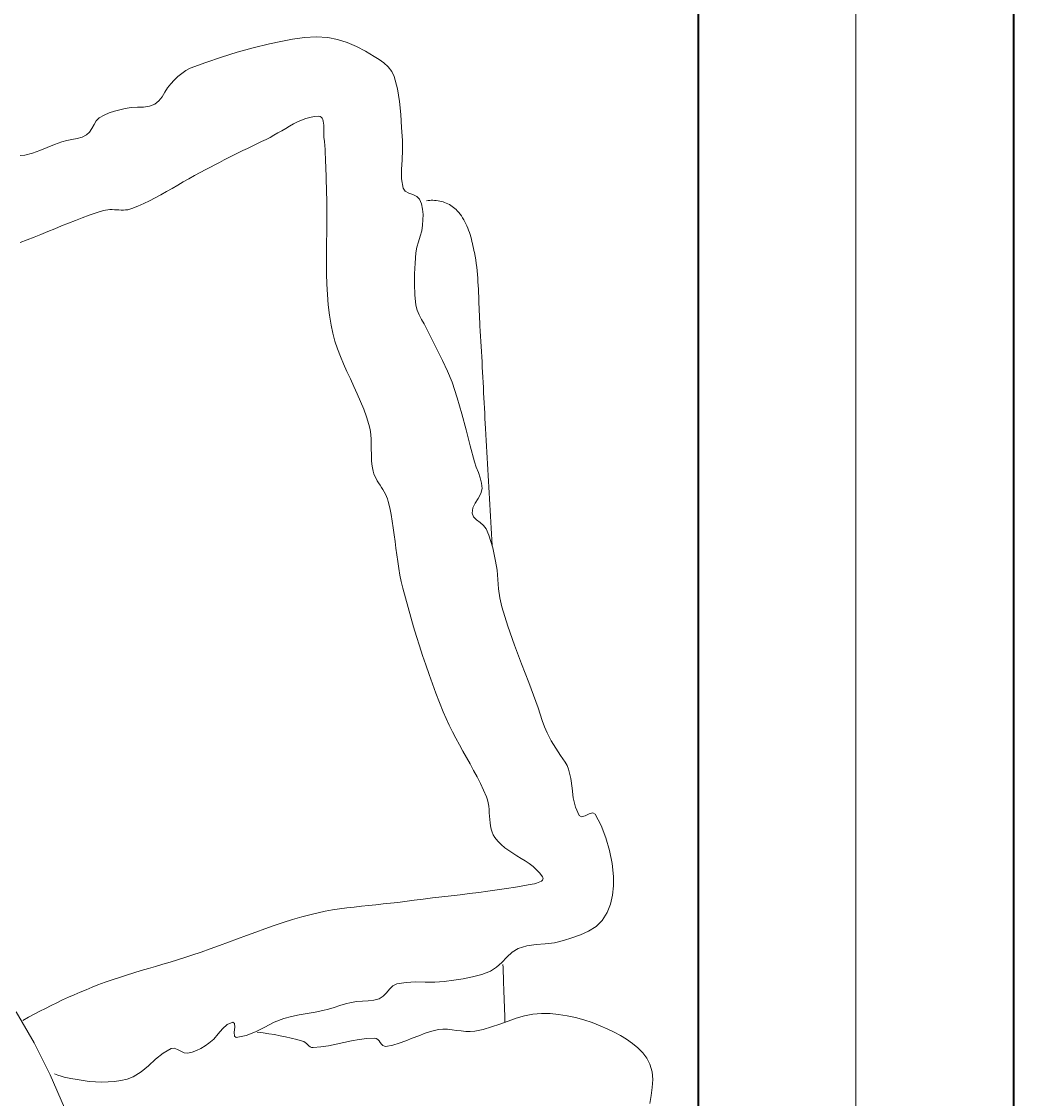
# Model space of a CAD drawing. Units: inches. Extents: x 1441 to 2460, y 1648 to 2683.
# Tile 18 of 35: x 1861 to 1890, y 2091 to 2122. Entities that reach past the tile are written whole.
import ezdxf

# ---------------------------------------------------------------- set-up
doc = ezdxf.new("R2010")
doc.units = ezdxf.units.IN
for name, color, linetype, lineweight in [('A-ANNO-DIMS', 2, 'Continuous', 18), ('A-FURN', 8, 'Continuous', 15), ('A-GLAZ', 4, 'Continuous', 18), ('A-WALL', 7, 'Continuous', 40)]:
    doc.layers.add(name, color=color, linetype=linetype, lineweight=lineweight)
doc.styles.get("Standard").update_dxf_attribs({"font": 'arial.ttf'})
doc.dimstyles.get("Standard").update_dxf_attribs({"dimtxt": 0.18, "dimasz": 0.18, "dimexe": 0.18, "dimexo": 0.0625, "dimgap": 0.09, "dimtad": 0, "dimtih": 1, "dimtoh": 1, "dimdec": 4, "dimzin": 0, "dimdsep": 46, "dimtxsty": 'Standard', "dimcen": 0.09, "dimadec": 0, "dimazin": 0, "dimtfac": 1, "dimtdec": 4, "dimtofl": 0, "dimtmove": 0, "dimatfit": 3, "dimfxl": 1, "dimtolj": 1, "dimtzin": 0, "dimarcsym": 0})

# ---------------------------------------------------------------- blocks, each defined once
blk = doc.blocks.new('BED-DOUBLE-PLAN')
for p, q in [((30.874, 90.983), (30.661, 90.921)), ((31.094, 91.001), (30.874, 90.983)), ((31.32, 90.99), (31.094, 91.001)), ((31.549, 90.959), (31.32, 90.99)), ((31.78, 90.922), (31.549, 90.959)), ((30.333, 90.717), (30.192, 90.579)), ((30.489, 90.832), (30.333, 90.717)), ((30.661, 90.921), (30.489, 90.832)), ((30.063, 90.425), (29.947, 90.257)), ((30.192, 90.579), (30.063, 90.425)), ((29.842, 90.082), (29.747, 89.903)), ((29.947, 90.257), (29.842, 90.082)), ((24.202, 89.666), (24.563, 89.771)), ((24.563, 89.771), (24.931, 89.844)), ((24.931, 89.844), (25.302, 89.885)), ((25.302, 89.885), (25.565, 89.887)), ((25.565, 89.887), (25.831, 89.859)), ((25.831, 89.859), (26.09, 89.797)), ((26.09, 89.797), (26.334, 89.698)), ((29.66, 89.724), (29.561, 89.501)), ((29.747, 89.903), (29.66, 89.724)), ((23.52, 89.361), (23.852, 89.529)), ((23.852, 89.529), (24.202, 89.666)), ((26.334, 89.698), (26.554, 89.56)), ((26.554, 89.56), (26.727, 89.384)), ((29.561, 89.501), (29.471, 89.271)), ((23.486, 89.292), (23.52, 89.361)), ((23.516, 89.189), (23.486, 89.292)), ((23.569, 89.075), (23.516, 89.189)), ((26.727, 89.384), (26.861, 89.173)), ((26.861, 89.173), (26.965, 88.94)), ((29.471, 89.271), (29.393, 89.037)), ((23.32, 88.794), (23.566, 88.9)), ((23.566, 88.9), (23.6, 88.971)), ((23.6, 88.971), (23.569, 89.075)), ((26.965, 88.94), (27.052, 88.696)), ((29.327, 88.8), (29.274, 88.559)), ((29.393, 89.037), (29.327, 88.8)), ((21.942, 88.434), (22.037, 88.5)), ((22.037, 88.5), (22.136, 88.557)), ((22.136, 88.557), (22.241, 88.602)), ((22.241, 88.602), (22.507, 88.665)), ((22.507, 88.665), (22.781, 88.701)), ((22.781, 88.701), (23.055, 88.736)), ((23.055, 88.736), (23.32, 88.794)), ((27.052, 88.696), (27.132, 88.454)), ((29.274, 88.559), (29.236, 88.317)), ((21.536, 88.173), (21.643, 88.24)), ((21.643, 88.24), (21.75, 88.305)), ((21.75, 88.305), (21.847, 88.368)), ((21.847, 88.368), (21.942, 88.434)), ((27.132, 88.454), (27.192, 88.199)), ((27.192, 88.199), (27.223, 87.936)), ((29.236, 88.317), (29.214, 88.073)), ((20.851, 87.851), (21.031, 87.917)), ((21.031, 87.917), (21.207, 87.99)), ((21.207, 87.99), (21.32, 88.045)), ((21.32, 88.045), (21.429, 88.107)), ((21.429, 88.107), (21.536, 88.173)), ((27.223, 87.936), (27.246, 87.672)), ((29.214, 88.073), (29.208, 87.829)), ((19.771, 87.466), (20.309, 87.666)), ((20.309, 87.666), (20.489, 87.729)), ((20.489, 87.729), (20.67, 87.789)), ((20.67, 87.789), (20.851, 87.851)), ((24.936, 87.481), (25.019, 87.589)), ((25.019, 87.589), (25.108, 87.69)), ((25.108, 87.69), (25.206, 87.78)), ((25.206, 87.78), (25.316, 87.859)), ((25.316, 87.859), (25.351, 87.873)), ((25.351, 87.873), (25.382, 87.87)), ((25.382, 87.87), (25.41, 87.854)), ((25.41, 87.854), (25.435, 87.824)), ((25.435, 87.824), (25.457, 87.785)), ((25.457, 87.785), (25.476, 87.737)), ((25.476, 87.737), (25.493, 87.683)), ((25.493, 87.683), (25.508, 87.626)), ((25.508, 87.626), (25.521, 87.566)), ((27.246, 87.672), (27.284, 87.412)), ((29.208, 87.829), (29.229, 87.585)), ((29.229, 87.585), (29.278, 87.345)), ((19.236, 87.259), (19.771, 87.466)), ((24.785, 87.248), (24.859, 87.366)), ((24.859, 87.366), (24.936, 87.481)), ((25.521, 87.566), (25.532, 87.506)), ((25.532, 87.506), (25.542, 87.449)), ((25.542, 87.449), (25.551, 87.396)), ((25.551, 87.396), (25.559, 87.349)), ((25.559, 87.349), (25.604, 87.088)), ((27.284, 87.412), (27.359, 87.162)), ((29.278, 87.345), (29.347, 87.108)), ((18.16, 86.865), (18.7, 87.056)), ((18.7, 87.056), (19.236, 87.259)), ((24.562, 86.894), (24.638, 87.01)), ((24.638, 87.01), (24.712, 87.129)), ((24.712, 87.129), (24.785, 87.248)), ((25.604, 87.088), (25.646, 86.826)), ((27.359, 87.162), (27.462, 86.991)), ((27.462, 86.991), (27.601, 86.84)), ((29.347, 87.108), (29.428, 86.873)), ((17.356, 86.638), (17.613, 86.694)), ((17.613, 86.694), (18.16, 86.865)), ((24.299, 86.583), (24.394, 86.678)), ((24.394, 86.678), (24.481, 86.782)), ((24.481, 86.782), (24.562, 86.894)), ((25.646, 86.826), (25.684, 86.564)), ((27.601, 86.84), (27.752, 86.698)), ((27.752, 86.698), (27.893, 86.548)), ((27.813, 86.729), (27.896, 86.732)), ((27.896, 86.732), (27.979, 86.735)), ((27.979, 86.735), (28.061, 86.738)), ((28.061, 86.738), (28.144, 86.741)), ((28.144, 86.741), (28.226, 86.744)), ((28.226, 86.744), (28.309, 86.746)), ((28.309, 86.746), (28.391, 86.749)), ((28.391, 86.749), (28.474, 86.752)), ((28.474, 86.752), (28.556, 86.755)), ((28.556, 86.755), (28.639, 86.758)), ((28.639, 86.758), (28.722, 86.761)), ((28.722, 86.761), (28.804, 86.764)), ((28.804, 86.764), (28.887, 86.767)), ((28.887, 86.767), (28.969, 86.77)), ((28.969, 86.77), (29.052, 86.772)), ((29.052, 86.772), (29.134, 86.775)), ((29.134, 86.775), (29.217, 86.778)), ((29.217, 86.778), (29.3, 86.781)), ((29.3, 86.781), (29.382, 86.784)), ((29.382, 86.784), (29.465, 86.787)), ((29.428, 86.873), (29.514, 86.638)), ((14.359, 86.335), (14.526, 86.344)), ((14.526, 86.344), (14.693, 86.354)), ((14.693, 86.354), (14.859, 86.363)), ((14.859, 86.363), (15.026, 86.373)), ((15.026, 86.373), (15.193, 86.382)), ((15.193, 86.382), (15.36, 86.392)), ((15.36, 86.392), (15.527, 86.401)), ((15.527, 86.401), (15.694, 86.411)), ((15.56, 86.325), (15.741, 86.387)), ((15.694, 86.411), (15.86, 86.42)), ((15.741, 86.387), (15.927, 86.438)), ((15.927, 86.438), (16.114, 86.481)), ((16.114, 86.481), (16.302, 86.52)), ((16.302, 86.52), (16.564, 86.559)), ((16.564, 86.559), (16.828, 86.583)), ((16.828, 86.583), (17.093, 86.605)), ((17.093, 86.605), (17.356, 86.638)), ((23.389, 86.334), (23.483, 86.34)), ((23.483, 86.34), (23.578, 86.346)), ((23.578, 86.346), (23.673, 86.352)), ((23.673, 86.352), (23.767, 86.361)), ((23.767, 86.361), (23.858, 86.373)), ((23.858, 86.373), (23.948, 86.391)), ((23.948, 86.391), (24.034, 86.417)), ((24.034, 86.417), (24.116, 86.452)), ((24.116, 86.452), (24.194, 86.499)), ((24.194, 86.499), (24.299, 86.583)), ((25.684, 86.564), (25.721, 86.301)), ((27.893, 86.548), (28, 86.378)), ((28, 86.378), (28.096, 86.124)), ((29.514, 86.638), (29.596, 86.402)), ((29.596, 86.402), (29.666, 86.164)), ((8.649, 86.032), (8.755, 86.037)), ((8.755, 86.037), (8.86, 86.04)), ((8.86, 86.04), (8.965, 86.044)), ((8.965, 86.044), (9.07, 86.048)), ((9.07, 86.048), (9.175, 86.052)), ((9.175, 86.052), (9.281, 86.056)), ((9.281, 86.056), (9.386, 86.061)), ((9.386, 86.061), (9.491, 86.066)), ((9.491, 86.066), (9.595, 86.072)), ((9.595, 86.072), (9.742, 86.081)), ((9.742, 86.081), (9.888, 86.09)), ((9.888, 86.09), (10.035, 86.099)), ((10.035, 86.099), (10.181, 86.107)), ((10.181, 86.107), (10.327, 86.116)), ((10.327, 86.116), (10.474, 86.124)), ((10.474, 86.124), (10.62, 86.132)), ((10.62, 86.132), (10.767, 86.14)), ((10.767, 86.14), (10.913, 86.147)), ((10.913, 86.147), (11.059, 86.155)), ((11.059, 86.155), (11.206, 86.163)), ((11.206, 86.163), (11.352, 86.17)), ((11.352, 86.17), (11.499, 86.178)), ((11.499, 86.178), (11.645, 86.185)), ((11.645, 86.185), (11.792, 86.193)), ((11.792, 86.193), (11.938, 86.201)), ((11.938, 86.201), (12.085, 86.209)), ((12.085, 86.209), (12.231, 86.216)), ((12.231, 86.216), (12.377, 86.224)), ((12.377, 86.224), (12.524, 86.232)), ((12.524, 86.232), (12.691, 86.242)), ((12.691, 86.242), (12.858, 86.251)), ((12.858, 86.251), (13.024, 86.26)), ((13.024, 86.26), (13.191, 86.27)), ((13.191, 86.27), (13.358, 86.279)), ((13.358, 86.279), (13.525, 86.288)), ((13.525, 86.288), (13.692, 86.298)), ((13.692, 86.298), (13.859, 86.307)), ((13.774, 86.028), (13.925, 86.082)), ((13.859, 86.307), (14.025, 86.316)), ((13.925, 86.082), (14.077, 86.121)), ((14.025, 86.316), (14.192, 86.326)), ((14.077, 86.121), (14.232, 86.132)), ((14.192, 86.326), (14.359, 86.335)), ((14.232, 86.132), (14.378, 86.095)), ((14.378, 86.095), (14.515, 86.019)), ((15.126, 85.971), (15.205, 86.075)), ((15.205, 86.075), (15.287, 86.175)), ((15.287, 86.175), (15.385, 86.249)), ((15.385, 86.249), (15.56, 86.325)), ((22.459, 85.991), (22.646, 86.085)), ((22.646, 86.085), (22.835, 86.174)), ((22.835, 86.174), (23.026, 86.257)), ((23.026, 86.257), (23.113, 86.287)), ((23.113, 86.287), (23.203, 86.309)), ((23.203, 86.309), (23.295, 86.324)), ((23.295, 86.324), (23.389, 86.334)), ((25.721, 86.301), (25.756, 86.038)), ((25.756, 86.038), (25.789, 85.775)), ((28.096, 86.124), (28.167, 85.862)), ((29.666, 86.164), (29.717, 85.922)), ((6.802, 85.724), (6.864, 85.748)), ((6.864, 85.748), (6.926, 85.77)), ((6.926, 85.77), (6.989, 85.79)), ((6.989, 85.79), (7.053, 85.809)), ((7.053, 85.809), (7.117, 85.827)), ((7.117, 85.827), (7.181, 85.844)), ((7.181, 85.844), (7.246, 85.86)), ((7.246, 85.86), (7.31, 85.874)), ((7.31, 85.874), (7.374, 85.888)), ((7.374, 85.888), (7.438, 85.902)), ((7.438, 85.902), (7.502, 85.915)), ((7.502, 85.915), (7.605, 85.934)), ((7.605, 85.934), (7.709, 85.951)), ((7.709, 85.951), (7.812, 85.966)), ((7.812, 85.966), (7.916, 85.979)), ((7.916, 85.979), (8.021, 85.99)), ((8.021, 85.99), (8.125, 86)), ((8.125, 86), (8.23, 86.008)), ((8.23, 86.008), (8.334, 86.016)), ((8.334, 86.016), (8.439, 86.022)), ((8.439, 86.022), (8.544, 86.028)), ((8.544, 86.028), (8.649, 86.032)), ((12.558, 85.676), (13.016, 85.794)), ((13.016, 85.794), (13.473, 85.918)), ((13.473, 85.918), (13.624, 85.969)), ((13.624, 85.969), (13.774, 86.028)), ((14.515, 86.019), (14.65, 85.933)), ((14.65, 85.933), (14.788, 85.865)), ((14.788, 85.865), (14.932, 85.847)), ((14.932, 85.847), (15.039, 85.888)), ((15.039, 85.888), (15.126, 85.971)), ((21.908, 85.69), (22.091, 85.792)), ((22.091, 85.792), (22.274, 85.893)), ((22.274, 85.893), (22.459, 85.991)), ((25.789, 85.775), (25.821, 85.511)), ((28.167, 85.862), (28.22, 85.594)), ((29.717, 85.922), (29.728, 85.794)), ((29.728, 85.794), (29.724, 85.665)), ((6.273, 85.391), (6.306, 85.423)), ((6.306, 85.423), (6.354, 85.466)), ((6.354, 85.466), (6.405, 85.506)), ((6.405, 85.506), (6.457, 85.544)), ((6.457, 85.544), (6.511, 85.579)), ((6.511, 85.579), (6.567, 85.612)), ((6.567, 85.612), (6.624, 85.643)), ((6.624, 85.643), (6.682, 85.672)), ((6.682, 85.672), (6.742, 85.699)), ((6.742, 85.699), (6.802, 85.724)), ((11.197, 85.276), (11.645, 85.425)), ((11.645, 85.425), (12.1, 85.556)), ((12.1, 85.556), (12.558, 85.676)), ((21.358, 85.385), (21.542, 85.485)), ((21.542, 85.485), (21.725, 85.587)), ((21.725, 85.587), (21.908, 85.69)), ((25.821, 85.511), (25.853, 85.248)), ((28.22, 85.594), (28.261, 85.323)), ((29.71, 85.536), (29.692, 85.406)), ((29.724, 85.665), (29.71, 85.536)), ((6.092, 85.111), (6.112, 85.155)), ((6.112, 85.155), (6.134, 85.199)), ((6.134, 85.199), (6.158, 85.24)), ((6.158, 85.24), (6.184, 85.281)), ((6.184, 85.281), (6.212, 85.319)), ((6.212, 85.319), (6.241, 85.356)), ((6.241, 85.356), (6.273, 85.391)), ((10.576, 85.005), (10.883, 85.149)), ((10.883, 85.149), (11.197, 85.276)), ((20.796, 85.106), (20.986, 85.194)), ((20.986, 85.194), (21.173, 85.287)), ((21.173, 85.287), (21.358, 85.385)), ((25.853, 85.248), (25.884, 84.984)), ((28.261, 85.323), (28.298, 85.053)), ((29.661, 85.147), (29.658, 85.018)), ((29.674, 85.276), (29.661, 85.147)), ((29.692, 85.406), (29.674, 85.276)), ((6.011, 84.78), (6.015, 84.828)), ((6.015, 84.828), (6.023, 84.877)), ((6.023, 84.877), (6.032, 84.924)), ((6.032, 84.924), (6.044, 84.972)), ((6.044, 84.972), (6.057, 85.019)), ((6.057, 85.019), (6.073, 85.065)), ((6.073, 85.065), (6.092, 85.111)), ((9.972, 84.695), (10.274, 84.851)), ((10.274, 84.851), (10.576, 85.005)), ((19.804, 84.719), (20.072, 84.818)), ((20.072, 84.818), (20.338, 84.92)), ((20.338, 84.92), (20.604, 85.025)), ((20.604, 85.025), (20.796, 85.106)), ((25.884, 84.984), (25.915, 84.72)), ((28.298, 85.053), (28.318, 84.783)), ((29.658, 85.018), (29.671, 84.89)), ((29.671, 84.89), (29.714, 84.699)), ((6.009, 84.732), (6.011, 84.78)), ((6.009, 84.685), (6.009, 84.732)), ((6.012, 84.638), (6.009, 84.685)), ((6.017, 84.591), (6.012, 84.638)), ((6.025, 84.546), (6.017, 84.591)), ((9.537, 84.478), (9.668, 84.546)), ((9.668, 84.546), (9.972, 84.695)), ((18.995, 84.438), (19.265, 84.529)), ((19.265, 84.529), (19.535, 84.623)), ((19.535, 84.623), (19.804, 84.719)), ((25.915, 84.72), (25.948, 84.457)), ((28.316, 84.51), (28.311, 84.238)), ((28.318, 84.783), (28.316, 84.51)), ((29.714, 84.699), (29.774, 84.511)), ((29.774, 84.511), (29.844, 84.326)), ((5.848, 84.161), (5.898, 84.271)), ((5.898, 84.271), (5.976, 84.349)), ((5.976, 84.349), (6.115, 84.405)), ((6.115, 84.405), (6.262, 84.436)), ((6.262, 84.436), (6.415, 84.448)), ((6.415, 84.448), (6.569, 84.447)), ((6.569, 84.447), (6.721, 84.438)), ((6.721, 84.438), (6.88, 84.413)), ((6.88, 84.413), (7.036, 84.368)), ((7.036, 84.368), (7.192, 84.317)), ((7.192, 84.317), (7.348, 84.271)), ((7.348, 84.271), (7.507, 84.244)), ((7.507, 84.244), (7.806, 84.221)), ((7.806, 84.221), (8.105, 84.206)), ((8.105, 84.206), (8.405, 84.203)), ((8.405, 84.203), (8.703, 84.214)), ((8.703, 84.214), (9, 84.245)), ((9, 84.245), (9.141, 84.279)), ((9.141, 84.279), (9.276, 84.335)), ((9.276, 84.335), (9.407, 84.405)), ((9.407, 84.405), (9.537, 84.478)), ((18.177, 84.181), (18.451, 84.264)), ((18.451, 84.264), (18.723, 84.35)), ((18.723, 84.35), (18.995, 84.438)), ((25.948, 84.457), (25.981, 84.194)), ((25.981, 84.194), (26.015, 83.931)), ((28.311, 84.238), (28.322, 83.968)), ((29.844, 84.326), (29.919, 84.142)), ((5.668, 83.879), (5.753, 83.94)), ((5.753, 83.94), (5.807, 84.042)), ((5.807, 84.042), (5.848, 84.161)), ((17.078, 83.873), (17.353, 83.946)), ((17.353, 83.946), (17.629, 84.022)), ((17.629, 84.022), (17.903, 84.1)), ((17.903, 84.1), (18.177, 84.181)), ((26.015, 83.931), (26.042, 83.725)), ((28.322, 83.968), (28.367, 83.704)), ((29.919, 84.142), (29.993, 83.958)), ((29.993, 83.958), (30.06, 83.772)), ((2.331, 83.555), (2.475, 83.624)), ((2.475, 83.624), (2.83, 83.719)), ((2.83, 83.719), (3.193, 83.779)), ((3.193, 83.779), (3.561, 83.814)), ((3.561, 83.814), (3.931, 83.839)), ((3.931, 83.839), (4.3, 83.864)), ((4.3, 83.864), (4.575, 83.867)), ((4.575, 83.867), (4.852, 83.849)), ((4.852, 83.849), (5.128, 83.83)), ((5.128, 83.83), (5.401, 83.833)), ((5.401, 83.833), (5.668, 83.879)), ((15.168, 83.572), (15.359, 83.6)), ((15.359, 83.6), (15.551, 83.626)), ((15.551, 83.626), (15.743, 83.651)), ((15.743, 83.651), (15.935, 83.675)), ((15.935, 83.675), (16.128, 83.699)), ((16.128, 83.699), (16.319, 83.726)), ((16.319, 83.726), (16.51, 83.755)), ((16.51, 83.755), (16.701, 83.789)), ((16.701, 83.789), (16.89, 83.828)), ((16.89, 83.828), (17.078, 83.873)), ((26.042, 83.725), (26.065, 83.518)), ((28.367, 83.704), (28.424, 83.589)), ((28.424, 83.589), (28.516, 83.493)), ((30.06, 83.772), (30.115, 83.584)), ((30.115, 83.584), (30.152, 83.392)), ((1.99, 83.199), (2.089, 83.333)), ((2.089, 83.333), (2.203, 83.455)), ((2.203, 83.455), (2.331, 83.555)), ((14.201, 83.262), (14.265, 83.302)), ((14.265, 83.302), (14.329, 83.341)), ((14.329, 83.341), (14.394, 83.376)), ((14.394, 83.376), (14.461, 83.408)), ((14.461, 83.408), (14.529, 83.436)), ((14.529, 83.436), (14.6, 83.457)), ((14.6, 83.457), (14.788, 83.501)), ((14.788, 83.501), (14.977, 83.539)), ((14.977, 83.539), (15.168, 83.572)), ((26.065, 83.518), (26.087, 83.311)), ((26.087, 83.311), (26.108, 83.104)), ((28.516, 83.493), (28.62, 83.403)), ((28.62, 83.403), (28.718, 83.309)), ((28.718, 83.309), (28.788, 83.198)), ((30.121, 83.303), (30.083, 83.265)), ((30.146, 83.345), (30.121, 83.303)), ((30.152, 83.392), (30.146, 83.345)), ((1.759, 82.808), (1.902, 83.059)), ((1.902, 83.059), (1.99, 83.199)), ((12.711, 82.96), (12.814, 82.967)), ((12.814, 82.967), (12.917, 82.971)), ((12.917, 82.971), (13.021, 82.972)), ((13.021, 82.972), (13.125, 82.973)), ((13.125, 82.973), (13.229, 82.974)), ((13.229, 82.974), (13.332, 82.976)), ((13.332, 82.976), (13.435, 82.982)), ((13.435, 82.982), (13.538, 82.991)), ((13.538, 82.991), (13.639, 83.006)), ((13.639, 83.006), (13.739, 83.027)), ((13.739, 83.027), (13.81, 83.049)), ((13.81, 83.049), (13.878, 83.076)), ((13.878, 83.076), (13.945, 83.108)), ((13.945, 83.108), (14.01, 83.144)), ((14.01, 83.144), (14.074, 83.182)), ((14.074, 83.182), (14.138, 83.222)), ((14.138, 83.222), (14.201, 83.262)), ((26.108, 83.104), (26.129, 82.897)), ((28.788, 83.198), (28.833, 83.045)), ((28.833, 83.045), (28.854, 82.886)), ((29.921, 83.113), (29.911, 83.066)), ((29.911, 83.066), (29.924, 82.845)), ((29.95, 83.155), (29.921, 83.113)), ((29.991, 83.193), (29.95, 83.155)), ((30.037, 83.229), (29.991, 83.193)), ((30.083, 83.265), (30.037, 83.229)), ((1.626, 82.55), (1.759, 82.808)), ((11.535, 82.573), (11.75, 82.667)), ((11.75, 82.667), (11.967, 82.755)), ((11.967, 82.755), (12.187, 82.836)), ((12.187, 82.836), (12.409, 82.906)), ((12.409, 82.906), (12.509, 82.931)), ((12.509, 82.931), (12.61, 82.948)), ((12.61, 82.948), (12.711, 82.96)), ((26.129, 82.897), (26.151, 82.689)), ((26.151, 82.689), (26.173, 82.483)), ((28.854, 82.886), (28.863, 82.724)), ((28.863, 82.724), (28.873, 82.561)), ((29.924, 82.845), (29.954, 82.626)), ((1.51, 82.285), (1.626, 82.55)), ((10.894, 82.279), (11.108, 82.377)), ((11.108, 82.377), (11.321, 82.476)), ((11.321, 82.476), (11.535, 82.573)), ((26.173, 82.483), (26.198, 82.276)), ((28.873, 82.561), (28.896, 82.401)), ((28.896, 82.401), (28.937, 82.237)), ((29.954, 82.626), (29.995, 82.407)), ((29.995, 82.407), (30.042, 82.189)), ((1.42, 82.012), (1.51, 82.285)), ((10.246, 82.01), (10.464, 82.093)), ((10.464, 82.093), (10.679, 82.183)), ((10.679, 82.183), (10.894, 82.279)), ((26.198, 82.276), (26.226, 82.07)), ((26.226, 82.07), (26.258, 81.865)), ((28.937, 82.237), (28.985, 82.075)), ((28.985, 82.075), (29.036, 81.914)), ((30.042, 82.189), (30.09, 81.971)), ((1.366, 81.731), (1.42, 82.012)), ((8.697, 81.719), (8.991, 81.743)), ((8.991, 81.743), (9.283, 81.778)), ((9.283, 81.778), (9.574, 81.824)), ((9.574, 81.824), (9.802, 81.873)), ((9.802, 81.873), (10.026, 81.936)), ((10.026, 81.936), (10.246, 82.01)), ((26.258, 81.865), (26.294, 81.661)), ((29.036, 81.914), (29.086, 81.753)), ((29.086, 81.753), (29.129, 81.589)), ((30.09, 81.971), (30.133, 81.753)), ((30.133, 81.753), (30.166, 81.534)), ((1.348, 81.397), (1.366, 81.731)), ((3.612, 81.466), (3.617, 81.509)), ((3.623, 81.342), (3.612, 81.466)), ((3.617, 81.509), (3.635, 81.543)), ((3.635, 81.543), (3.665, 81.569)), ((3.665, 81.569), (3.704, 81.588)), ((3.704, 81.588), (3.751, 81.602)), ((3.751, 81.602), (3.804, 81.61)), ((3.804, 81.61), (3.862, 81.615)), ((3.862, 81.615), (3.922, 81.618)), ((3.922, 81.618), (3.984, 81.618)), ((3.984, 81.618), (4.046, 81.618)), ((4.046, 81.618), (4.106, 81.618)), ((4.106, 81.618), (4.162, 81.619)), ((4.162, 81.619), (4.212, 81.623)), ((4.212, 81.623), (4.329, 81.634)), ((4.329, 81.634), (4.446, 81.644)), ((4.446, 81.644), (4.564, 81.652)), ((4.564, 81.652), (4.681, 81.659)), ((4.681, 81.659), (4.798, 81.665)), ((4.798, 81.665), (4.916, 81.67)), ((4.916, 81.67), (5.033, 81.674)), ((5.033, 81.674), (5.151, 81.678)), ((5.151, 81.678), (5.269, 81.681)), ((5.269, 81.681), (5.386, 81.684)), ((5.386, 81.684), (5.504, 81.688)), ((5.504, 81.688), (5.621, 81.691)), ((5.621, 81.691), (5.739, 81.695)), ((5.739, 81.695), (6.034, 81.703)), ((6.034, 81.703), (6.33, 81.706)), ((6.33, 81.706), (6.626, 81.704)), ((6.626, 81.704), (6.923, 81.701)), ((6.923, 81.701), (7.219, 81.696)), ((7.219, 81.696), (7.516, 81.693)), ((7.516, 81.693), (7.812, 81.692)), ((7.812, 81.692), (8.108, 81.695)), ((8.108, 81.695), (8.403, 81.703)), ((8.403, 81.703), (8.697, 81.719)), ((26.294, 81.661), (26.335, 81.458)), ((26.335, 81.458), (26.383, 81.256)), ((29.129, 81.589), (29.175, 81.367)), ((30.166, 81.534), (30.185, 81.313)), ((1.367, 81.062), (1.348, 81.397)), ((3.646, 81.22), (3.623, 81.342)), ((3.68, 81.101), (3.646, 81.22)), ((26.383, 81.256), (26.454, 80.989)), ((29.175, 81.367), (29.213, 81.142)), ((29.213, 81.142), (29.25, 80.917)), ((30.071, 81.123), (30.04, 81.086)), ((30.104, 81.158), (30.071, 81.123)), ((30.136, 81.194), (30.104, 81.158)), ((30.162, 81.231), (30.136, 81.194)), ((30.179, 81.27), (30.162, 81.231)), ((30.185, 81.313), (30.179, 81.27)), ((1.413, 80.727), (1.367, 81.062)), ((3.723, 80.984), (3.68, 81.101)), ((3.774, 80.869), (3.723, 80.984)), ((3.831, 80.755), (3.774, 80.869)), ((26.454, 80.989), (26.531, 80.724)), ((29.25, 80.917), (29.294, 80.695)), ((29.954, 80.848), (29.915, 80.689)), ((29.996, 81.006), (29.954, 80.848)), ((30.014, 81.048), (29.996, 81.006)), ((30.04, 81.086), (30.014, 81.048)), ((1.477, 80.394), (1.413, 80.727)), ((3.892, 80.643), (3.831, 80.755)), ((3.957, 80.531), (3.892, 80.643)), ((4.023, 80.419), (3.957, 80.531)), ((26.531, 80.724), (26.614, 80.46)), ((29.294, 80.695), (29.352, 80.475)), ((29.879, 80.529), (29.846, 80.368)), ((29.915, 80.689), (29.879, 80.529)), ((1.549, 80.065), (1.477, 80.394)), ((4.088, 80.308), (4.023, 80.419)), ((4.153, 80.196), (4.088, 80.308)), ((4.214, 80.084), (4.153, 80.196)), ((26.614, 80.46), (26.702, 80.198)), ((26.702, 80.198), (26.793, 79.936)), ((29.352, 80.475), (29.461, 80.202)), ((29.461, 80.202), (29.597, 79.937)), ((29.815, 80.207), (29.788, 80.045)), ((29.846, 80.368), (29.815, 80.207)), ((1.659, 79.605), (1.549, 80.065)), ((4.27, 79.971), (4.214, 80.084)), ((4.334, 79.837), (4.27, 79.971)), ((26.793, 79.936), (26.887, 79.676)), ((29.597, 79.937), (29.734, 79.673)), ((29.788, 80.045), (29.764, 79.883)), ((1.783, 79.148), (1.659, 79.605)), ((4.398, 79.704), (4.334, 79.837)), ((4.462, 79.571), (4.398, 79.704)), ((26.887, 79.676), (26.983, 79.416)), ((29.734, 79.673), (29.843, 79.403)), ((29.764, 79.883), (29.743, 79.721)), ((4.527, 79.438), (4.462, 79.571)), ((4.593, 79.305), (4.527, 79.438)), ((4.659, 79.173), (4.593, 79.305)), ((26.983, 79.416), (27.08, 79.157)), ((29.843, 79.403), (29.9, 79.12)), ((1.921, 78.696), (1.783, 79.148)), ((4.725, 79.041), (4.659, 79.173)), ((4.792, 78.909), (4.725, 79.041)), ((27.08, 79.157), (27.177, 78.897)), ((29.494, 79.073), (29.458, 79.021)), ((29.458, 79.021), (29.528, 78.86)), ((29.604, 79.076), (29.494, 79.073)), ((29.741, 79.063), (29.604, 79.076)), ((29.856, 79.066), (29.741, 79.063)), ((29.9, 79.12), (29.856, 79.066)), ((2.075, 78.248), (1.921, 78.696)), ((4.859, 78.777), (4.792, 78.909)), ((4.927, 78.645), (4.859, 78.777)), ((27.177, 78.897), (27.274, 78.638)), ((29.528, 78.86), (29.648, 78.726)), ((29.648, 78.726), (29.793, 78.603)), ((4.994, 78.513), (4.927, 78.645)), ((5.062, 78.382), (4.994, 78.513)), ((5.13, 78.25), (5.062, 78.382)), ((27.274, 78.638), (27.368, 78.377)), ((27.368, 78.377), (27.461, 78.116)), ((29.793, 78.603), (29.939, 78.48)), ((29.939, 78.48), (30.061, 78.342)), ((2.244, 77.807), (2.075, 78.248)), ((5.215, 78.088), (5.13, 78.25)), ((5.304, 77.927), (5.215, 78.088)), ((27.461, 78.116), (27.55, 77.854)), ((30.061, 78.342), (30.137, 78.228)), ((30.137, 78.228), (30.206, 78.109)), ((30.206, 78.109), (30.267, 77.986)), ((2.307, 77.68), (2.244, 77.807)), ((5.394, 77.767), (5.304, 77.927)), ((5.485, 77.608), (5.394, 77.767)), ((27.55, 77.854), (27.616, 77.649)), ((30.267, 77.986), (30.314, 77.859)), ((30.314, 77.859), (30.343, 77.727)), ((2.388, 77.564), (2.307, 77.68)), ((2.481, 77.454), (2.388, 77.564)), ((2.582, 77.35), (2.481, 77.454)), ((5.577, 77.449), (5.485, 77.608)), ((5.669, 77.289), (5.577, 77.449)), ((27.616, 77.649), (27.681, 77.442)), ((27.681, 77.442), (27.743, 77.235)), ((30.237, 77.443), (30.203, 77.351)), ((30.288, 77.537), (30.237, 77.443)), ((30.332, 77.631), (30.288, 77.537)), ((30.343, 77.727), (30.332, 77.631)), ((2.684, 77.249), (2.582, 77.35)), ((2.8, 77.157), (2.684, 77.249)), ((2.929, 77.079), (2.8, 77.157)), ((5.759, 77.13), (5.669, 77.289)), ((5.849, 76.969), (5.759, 77.13)), ((27.743, 77.235), (27.805, 77.028)), ((30.203, 77.351), (30.212, 77.262)), ((30.212, 77.262), (30.347, 77.03)), ((3.059, 77.002), (2.929, 77.079)), ((3.175, 76.914), (3.059, 77.002)), ((3.263, 76.801), (3.175, 76.914)), ((5.936, 76.808), (5.849, 76.969)), ((27.805, 77.028), (27.866, 76.82)), ((27.866, 76.82), (27.927, 76.612)), ((30.347, 77.03), (30.518, 76.819)), ((30.518, 76.819), (30.704, 76.617)), ((3.323, 76.643), (3.263, 76.801)), ((3.348, 76.473), (3.323, 76.643)), ((6.02, 76.645), (5.936, 76.808)), ((6.1, 76.48), (6.02, 76.645)), ((27.927, 76.612), (27.988, 76.405)), ((30.704, 76.617), (30.879, 76.408)), ((3.356, 76.298), (3.348, 76.473)), ((3.364, 76.122), (3.356, 76.298)), ((6.176, 76.314), (6.1, 76.48)), ((6.247, 76.145), (6.176, 76.314)), ((27.988, 76.405), (28.051, 76.197)), ((30.879, 76.408), (31.02, 76.18)), ((3.391, 75.951), (3.364, 76.122)), ((3.428, 75.797), (3.391, 75.951)), ((6.267, 76.086), (6.247, 76.145)), ((6.28, 76.025), (6.267, 76.086)), ((6.286, 75.963), (6.28, 76.025)), ((6.289, 75.9), (6.286, 75.963)), ((6.288, 75.836), (6.289, 75.9)), ((28.051, 76.197), (28.114, 75.991)), ((28.114, 75.991), (28.18, 75.785)), ((31.02, 76.18), (31.086, 76.009)), ((31.086, 76.009), (31.127, 75.831)), ((3.469, 75.643), (3.428, 75.797)), ((3.518, 75.492), (3.469, 75.643)), ((6.275, 75.579), (6.277, 75.643)), ((6.277, 75.643), (6.281, 75.708)), ((6.281, 75.708), (6.285, 75.772)), ((6.285, 75.772), (6.288, 75.836)), ((28.18, 75.785), (28.249, 75.58)), ((31.127, 75.831), (31.15, 75.647)), ((31.15, 75.647), (31.161, 75.461)), ((3.579, 75.347), (3.518, 75.492)), ((3.657, 75.211), (3.579, 75.347)), ((6.275, 75.515), (6.275, 75.579)), ((6.279, 75.452), (6.275, 75.515)), ((6.288, 75.39), (6.279, 75.452)), ((6.303, 75.329), (6.288, 75.39)), ((6.367, 75.127), (6.303, 75.329)), ((28.249, 75.58), (28.321, 75.376)), ((28.321, 75.376), (28.397, 75.174)), ((31.161, 75.461), (31.167, 75.277)), ((3.742, 75.126), (3.657, 75.211)), ((3.848, 75.061), (3.742, 75.126)), ((3.96, 75.003), (3.848, 75.061)), ((4.064, 74.937), (3.96, 75.003)), ((6.436, 74.927), (6.367, 75.127)), ((28.397, 75.174), (28.463, 75.004)), ((28.463, 75.004), (28.532, 74.835)), ((31.164, 75.101), (31.148, 74.926)), ((31.167, 75.277), (31.164, 75.101)), ((4.146, 74.85), (4.064, 74.937)), ((4.21, 74.72), (4.146, 74.85)), ((4.25, 74.579), (4.21, 74.72)), ((6.508, 74.728), (6.436, 74.927)), ((6.584, 74.53), (6.508, 74.728)), ((28.532, 74.835), (28.602, 74.666)), ((28.602, 74.666), (28.675, 74.499)), ((31.124, 74.751), (31.094, 74.577)), ((31.148, 74.926), (31.124, 74.751)), ((4.278, 74.433), (4.25, 74.579)), ((4.304, 74.287), (4.278, 74.433)), ((6.661, 74.333), (6.584, 74.53)), ((28.675, 74.499), (28.749, 74.332)), ((31.064, 74.403), (31.045, 74.308)), ((31.094, 74.577), (31.064, 74.403)), ((4.341, 74.144), (4.304, 74.287)), ((4.419, 73.932), (4.341, 74.144)), ((6.74, 74.136), (6.661, 74.333)), ((6.821, 73.94), (6.74, 74.136)), ((28.749, 74.332), (28.825, 74.166)), ((28.825, 74.166), (28.903, 74.001)), ((31.901, 74.215), (30.964, 73.813)), ((30.996, 74.121), (30.966, 74.029)), ((31.023, 74.214), (30.996, 74.121)), ((31.045, 74.308), (31.023, 74.214)), ((4.506, 73.724), (4.419, 73.932)), ((6.901, 73.744), (6.821, 73.94)), ((6.982, 73.548), (6.901, 73.744)), ((28.903, 74.001), (28.983, 73.837)), ((28.983, 73.837), (29.064, 73.674)), ((30.964, 73.813), (30.052, 73.35)), ((30.966, 74.029), (30.933, 73.938)), ((4.592, 73.515), (4.506, 73.724)), ((4.667, 73.304), (4.592, 73.515)), ((7.062, 73.352), (6.982, 73.548)), ((29.064, 73.674), (29.148, 73.511)), ((29.148, 73.511), (29.233, 73.35)), ((4.722, 73.087), (4.667, 73.304)), ((7.14, 73.155), (7.062, 73.352)), ((7.216, 72.957), (7.14, 73.155)), ((30.052, 73.35), (29.164, 72.842)), ((29.233, 73.35), (29.32, 73.189)), ((29.32, 73.189), (29.409, 73.03)), ((4.732, 72.953), (4.722, 73.087))]:
    blk.add_line(p, q)
blk = doc.blocks.new('WIN-48-SASH')
blk.add_line((4.496, 48.001), (4.496, 0.001))
blk = doc.blocks.new('*D67')
at = {"layer": 'A-ANNO-DIMS', "color": 0, "lineweight": -2, "transparency": 16777216}
for p, q in [((1889.448, 2298.695), (1916.216, 2298.695)), ((1916.036, 2298.515), (1916.036, 2055.938)), ((1916.036, 1812.997), (1916.036, 2055.574)), ((1758.224, 1812.817), (1916.216, 1812.817))]:
    blk.add_line(p, q, dxfattribs=at)
at = {"layer": 'A-ANNO-DIMS', "color": 0, "transparency": 16777216}
for points in [[(1916.006, 2298.515), (1916.066, 2298.515), (1916.036, 2298.695)], [(1916.006, 1812.997), (1916.066, 1812.997), (1916.036, 1812.817)]]:
    blk.add_solid(points, dxfattribs=at)
at = {"layer": 'Defpoints', "color": 0, "transparency": 16777216}
for p in [(1889.386, 2298.695), (1916.036, 2298.695), (1758.161, 1812.817)]:
    blk.add_point(p, dxfattribs=at)
at = {"layer": 'A-ANNO-DIMS', "color": 0, "transparency": 16777216, "insert": (1916.036, 2055.756), "char_height": 0.18, "attachment_point": 5}
blk.add_mtext('\\A1;485.9', dxfattribs=at)

msp = doc.modelspace()

# ---------------------------------------------------------------- linework, layer by layer
at = {"layer": 'A-WALL'}
for p, q in [((1889.3859, 2298.6952), (1889.3859, 1834.1952)), ((1880.3859, 2153.1952), (1880.3859, 1834.1952))]:
    msp.add_line(p, q, dxfattribs=at)

# ---------------------------------------------------------------- block references
at = {"layer": 'A-FURN', "rotation": 270}
msp.add_blockref('BED-DOUBLE-PLAN', (1788.0907, 2122.7206), dxfattribs=at)
at = {"layer": 'A-GLAZ'}
msp.add_blockref('WIN-48-SASH', (1880.39, 2076.1074), dxfattribs=at)

# ---------------------------------------------------------------- dimensions: what is measured, and where the dimension line sits
at = {"layer": 'A-ANNO-DIMS'}
dim = msp.add_linear_dim(base=(1916.0359, 2298.6952), p1=(1758.1615, 1812.8171), p2=(1889.3859, 2298.6952), angle=90, dimstyle='Standard', override={"dimdec": 1, "dimlfac": 1, "dimrnd": 0, "dimzin": 0, "dimdsep": 46, "dimlunit": 2}, dxfattribs=at)
dim.commit()
dim.dimension.update_dxf_attribs({"geometry": '*D67', "text_midpoint": (1916.0359, 2055.7561)})

doc.saveas('drawing.dxf')
